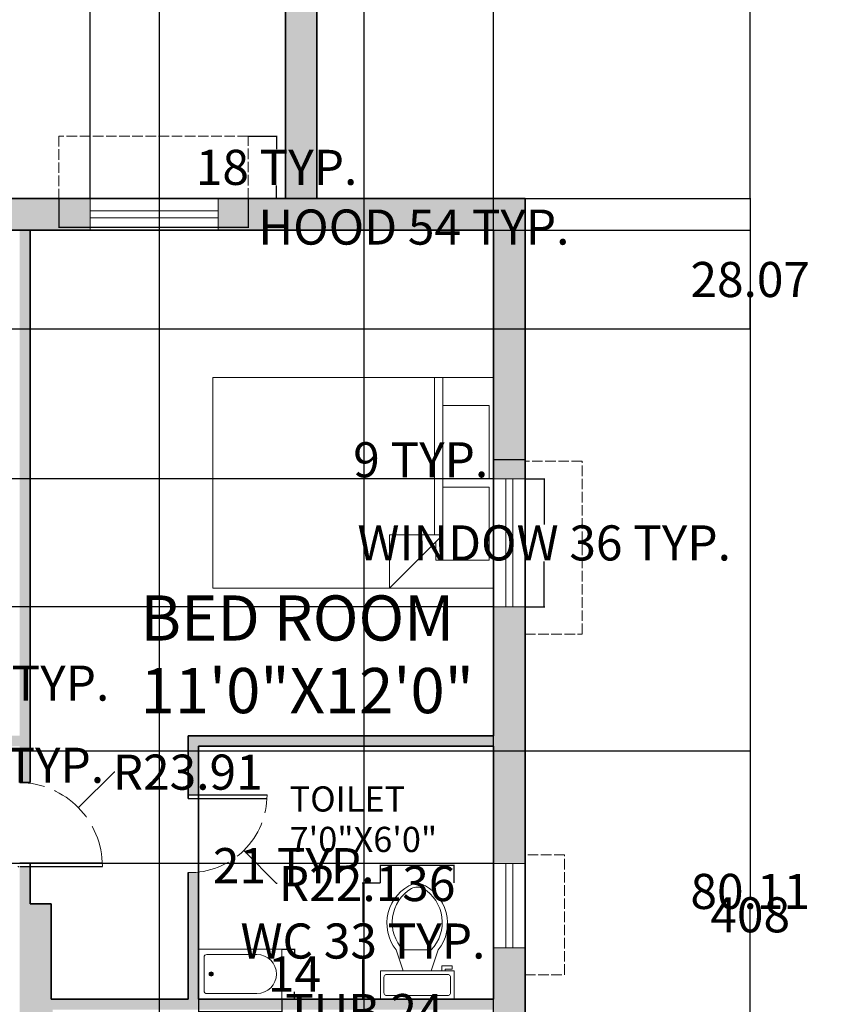
# Model space of a CAD drawing. Units: inches. Extents: x 300 to 1007, y 2 to 1069.
# Tile 7 of 12: x 766 to 995, y 253 to 533. Entities that reach past the tile are written whole.
import ezdxf

# ---------------------------------------------------------------- set-up
doc = ezdxf.new("R2010")
doc.units = ezdxf.units.IN
doc.header["$MEASUREMENT"] = 0
doc.linetypes.add('ACAD_ISO02W100', pattern=[15, 12, -3])
for name, color, linetype, lineweight in [('A-ANNO-DIMS', 2, 'Continuous', 18), ('A-AREA-IDEN', 7, 'Continuous', 18), ('A-DOOR', 3, 'Continuous', 25), ('A-DOOR-SWNG', 3, 'ACAD_ISO02W100', 13), ('A-FLOR-FIXT', 9, 'Continuous', 18), ('A-FLOR-SLAB', 7, 'Continuous', 35), ('A-FURN', 8, 'Continuous', 18), ('A-GLAZ', 4, 'Continuous', 18), ('A-GLAZ-OVHD', 8, 'ACAD_ISO02W100', 13), ('A-WALL', 7, 'Continuous', 35)]:
    doc.layers.add(name, color=color, linetype=linetype, lineweight=lineweight)
doc.layers.add('A-WALL-PATT', color=9, linetype='Continuous', lineweight=9, true_color=0xc7c8ca)
doc.styles.get("Standard").update_dxf_attribs({"font": 'arial.ttf'})
doc.dimstyles.get("Standard").update_dxf_attribs({"dimtxt": 10, "dimasz": 0.18, "dimexe": 0.18, "dimexo": 0.0625, "dimgap": 0.09, "dimtad": 0, "dimtih": 1, "dimtoh": 1, "dimdec": 0, "dimzin": 0, "dimdsep": 46, "dimlunit": 3, "dimtxsty": 'Standard', "dimcen": 0.09, "dimadec": 0, "dimazin": 0, "dimtfac": 1, "dimtdec": 0, "dimtofl": 0, "dimtmove": 0, "dimatfit": 3, "dimfxl": 1, "dimtolj": 1, "dimtzin": 0, "dimarcsym": 0})

# ---------------------------------------------------------------- blocks, each defined once
blk = doc.blocks.new('Bed - Queen')
for p, q in [((0, -80.00003), (0, 0)), ((0, 0), (59.99999, 0)), ((59.99999, 0), (59.99999, -80.00003)), ((7.99999, -1.2), (28.79998, -1.2)), ((7.99999, -14.4), (7.99999, -1.2)), ((28.79998, -1.2), (28.79998, -14.4)), ((31.19999, -1.2), (51.99999, -1.2)), ((31.19999, -14.4), (31.19999, -1.2)), ((51.99999, -1.2), (51.99999, -16.4)), ((0, -14.4), (44.8, -14.4)), ((44.8, -16.8), (0, -16.8)), ((59.99999, -29.6), (44.8, -14.4)), ((44.8, -14.4), (44.8, -29.6)), ((51.99999, -16.4), (46.79936, -16.4)), ((44.8, -29.6), (59.99999, -29.6)), ((59.99999, -80.00003), (0, -80.00003))]:
    blk.add_line(p, q)
blk = doc.blocks.new('Toilet - top')
for p, q in [((9.5, -6), (9.5, -2)), ((-8, -8.5), (-8, -8)), ((-7, -8), (-7, -9.5)), ((-4, -8), (-6, -14)), ((4, -8), (6, -14)), ((-10, -8.5), (-8, -8.5)), ((-10, -9.5), (-10, -8.5)), ((-7, -9.5), (-10, -9.5)), ((4, -14), (-4, -14))]:
    blk.add_line(p, q)
blk.add_lwpolyline([(10.5, -8), (10.5, 0), (-10.5, 0), (-10.5, -8)], close=True)
for points in [[(-9.5, -2), (-9.5, -6)], [(8.5, -1), (-8.5, -1)], [(-8.5, -7), (8.5, -7)]]:
    blk.add_lwpolyline(points)
for centre, radius, start, end in [((-8.62, -1.88), 0.884, 81.8699, 188.1301), ((8.62, -1.88), 0.884, 351.8699, 98.1301), ((-8.62, -6.12), 0.884, 171.8699, 278.1301), ((8.62, -6.12), 0.884, 261.8699, 8.1301), ((3.52, -21.58), 12.17, 141.4691, 247.9714), ((4.2, -21.82), 11.33, 136.3677, 238.9468), ((-3.52, -21.58), 12.17, 292.0284, 38.5307), ((-4.2, -21.82), 11.33, 301.053, 43.6321), ((0, -27.88), 4, 245.7318, 294.2682), ((0, -29), 4, 254.8605, 285.1395)]:
    blk.add_arc(centre, radius, start, end)
blk = doc.blocks.new('Bath Tub - 26 x 60 in.')
for p, q in [((8, -18), (10, -18)), ((9, -17), (9, -19))]:
    blk.add_line(p, q)
blk.add_lwpolyline([(0, -36), (0, 0), (60, 0), (60, -36)], close=True)
for points in [[(4, -30), (4, -6)], [(6, -4), (42, -4)], [(42, -32), (6, -32)]]:
    blk.add_lwpolyline(points)
for radius in [1.5, 1]:
    blk.add_circle((9, -18), radius)
for centre, radius, start, end in [((5.75, -5.75), 1.77, 81.8699, 188.1301), ((42, -18), 14, 270, 90), ((5.75, -30.25), 1.77, 171.8699, 278.1301)]:
    blk.add_arc(centre, radius, start, end)
blk = doc.blocks.new('WIN-24')
for p, q in [((0, -4.5), (0, 4.5)), ((23.96, 0), (23.96, 4.5)), ((23.96, 4.5), (23.96, -4.5)), ((0, 1), (23.96, 1)), ((0, -1), (23.96, -1))]:
    blk.add_line(p, q)
blk = doc.blocks.new('WIN-36_1-2')
for p, q in [((0, 4.5), (0, -4.5)), ((36.49, 0), (36.49, 4.5)), ((36.49, 4.5), (36.49, -4.5)), ((0, 1), (36.49, 1)), ((0, -1), (36.49, -1))]:
    blk.add_line(p, q)
blk = doc.blocks.new('WINDOW-HOOD-54')
at = {"ltscale": 0.25}
for p, q in [((0, 17.83), (-53.97, 17.83)), ((-53.97, 17.83), (-53.97, 0)), ((0, 0), (0, 17.83))]:
    blk.add_line(p, q, dxfattribs=at)
blk = doc.blocks.new('*D27')
at = {"layer": 'A-ANNO-DIMS', "color": 0, "lineweight": -2, "transparency": 16777216}
for p, q in [((777.25, 482.32), (777.25, 474.11)), ((831.22, 482.32), (831.22, 474.11)), ((777.43, 474.29), (831.04, 474.29)), ((831.22, 474.29), (831.4, 474.29))]:
    blk.add_line(p, q, dxfattribs=at)
at = {"layer": 'A-ANNO-DIMS', "color": 0, "transparency": 16777216}
for points in [[(777.43, 474.32), (777.43, 474.26), (777.25, 474.29)], [(831.04, 474.32), (831.04, 474.26), (831.22, 474.29)]]:
    blk.add_solid(points, dxfattribs=at)
at = {"layer": 'Defpoints', "color": 0, "transparency": 16777216}
for p in [(777.25, 482.38), (831.22, 482.38), (831.22, 474.29)]:
    blk.add_point(p, dxfattribs=at)
at = {"layer": 'A-ANNO-DIMS', "color": 0, "transparency": 16777216, "insert": (878.45, 474.29), "char_height": 10, "attachment_point": 5}
blk.add_mtext('\\A1;HOOD 54 TYP.', dxfattribs=at)
blk = doc.blocks.new('*D28')
at = {"layer": 'A-ANNO-DIMS', "color": 0, "lineweight": -2, "transparency": 16777216}
for p, q in [((831.28, 500.22), (839.5, 500.22)), ((839.32, 500.04), (839.32, 496.5)), ((839.32, 482.56), (839.32, 486.1)), ((831.28, 482.38), (839.5, 482.38))]:
    blk.add_line(p, q, dxfattribs=at)
at = {"layer": 'A-ANNO-DIMS', "color": 0, "transparency": 16777216}
for points in [[(839.29, 500.04), (839.35, 500.04), (839.32, 500.22)], [(839.29, 482.56), (839.35, 482.56), (839.32, 482.38)]]:
    blk.add_solid(points, dxfattribs=at)
at = {"layer": 'Defpoints', "color": 0, "transparency": 16777216}
for p in [(831.22, 500.22), (839.32, 500.22), (831.22, 482.38)]:
    blk.add_point(p, dxfattribs=at)
at = {"layer": 'A-ANNO-DIMS', "color": 0, "transparency": 16777216, "insert": (839.32, 491.3), "char_height": 10, "attachment_point": 5}
blk.add_mtext('\\A1;18 TYP.', dxfattribs=at)
blk = doc.blocks.new('*D31')
at = {"layer": 'A-ANNO-DIMS', "color": 0, "lineweight": -2, "transparency": 16777216}
for p, q in [((868.84, 287.43), (863.76, 287.43)), ((863.94, 287.25), (863.94, 276.17)), ((863.94, 254.56), (863.94, 265.64)), ((868.84, 254.38), (863.76, 254.38))]:
    blk.add_line(p, q, dxfattribs=at)
at = {"layer": 'A-ANNO-DIMS', "color": 0, "transparency": 16777216}
for points in [[(863.91, 287.25), (863.97, 287.25), (863.94, 287.43)], [(863.91, 254.56), (863.97, 254.56), (863.94, 254.38)]]:
    blk.add_solid(points, dxfattribs=at)
at = {"layer": 'Defpoints', "color": 0, "transparency": 16777216}
for p in [(868.9, 287.43), (863.94, 254.38), (868.9, 254.38)]:
    blk.add_point(p, dxfattribs=at)
at = {"layer": 'A-ANNO-DIMS', "color": 0, "transparency": 16777216, "insert": (863.94, 270.91), "char_height": 10, "attachment_point": 5}
blk.add_mtext('\\A1;WC 33 TYP.', dxfattribs=at)
blk = doc.blocks.new('*D32')
at = {"layer": 'A-ANNO-DIMS', "color": 0, "lineweight": -2, "transparency": 16777216}
for p, q in [((868.9, 292.39), (868.72, 292.39)), ((868.9, 287.49), (868.9, 292.57)), ((889.72, 292.39), (869.08, 292.39)), ((889.9, 287.49), (889.9, 292.57))]:
    blk.add_line(p, q, dxfattribs=at)
at = {"layer": 'A-ANNO-DIMS', "color": 0, "transparency": 16777216}
for points in [[(869.08, 292.42), (869.08, 292.36), (868.9, 292.39)], [(889.72, 292.42), (889.72, 292.36), (889.9, 292.39)]]:
    blk.add_solid(points, dxfattribs=at)
at = {"layer": 'Defpoints', "color": 0, "transparency": 16777216}
for p in [(868.9, 292.39), (868.9, 287.43), (889.9, 287.43)]:
    blk.add_point(p, dxfattribs=at)
at = {"layer": 'A-ANNO-DIMS', "color": 0, "transparency": 16777216, "insert": (844.2, 292.39), "char_height": 10, "attachment_point": 5}
blk.add_mtext('\\A1;21 TYP.', dxfattribs=at)
blk = doc.blocks.new('*D37')
at = {"layer": 'A-ANNO-DIMS', "color": 0, "lineweight": -2, "transparency": 16777216}
for p, q in [((817.12, 254.32), (817.12, 250.64)), ((840.87, 254.32), (840.87, 250.64)), ((817.3, 250.82), (840.69, 250.82)), ((840.87, 250.82), (841.05, 250.82))]:
    blk.add_line(p, q, dxfattribs=at)
at = {"layer": 'A-ANNO-DIMS', "color": 0, "transparency": 16777216}
for points in [[(817.3, 250.85), (817.3, 250.79), (817.12, 250.82)], [(840.69, 250.85), (840.69, 250.79), (840.87, 250.82)]]:
    blk.add_solid(points, dxfattribs=at)
at = {"layer": 'Defpoints', "color": 0, "transparency": 16777216}
for p in [(817.12, 254.38), (840.87, 254.38), (840.87, 250.82)]:
    blk.add_point(p, dxfattribs=at)
at = {"layer": 'A-ANNO-DIMS', "color": 0, "transparency": 16777216, "insert": (864.32, 250.82), "char_height": 10, "attachment_point": 5}
blk.add_mtext('\\A1;TUB 24', dxfattribs=at)
blk = doc.blocks.new('*D38')
at = {"layer": 'A-ANNO-DIMS', "color": 0, "lineweight": -2, "transparency": 16777216}
for p, q in [((840.93, 268.63), (844.61, 268.63)), ((844.43, 268.45), (844.43, 266.62)), ((844.43, 254.56), (844.43, 256.4)), ((840.93, 254.38), (844.61, 254.38))]:
    blk.add_line(p, q, dxfattribs=at)
at = {"layer": 'A-ANNO-DIMS', "color": 0, "transparency": 16777216}
for points in [[(844.4, 268.45), (844.46, 268.45), (844.43, 268.63)], [(844.4, 254.56), (844.46, 254.56), (844.43, 254.38)]]:
    blk.add_solid(points, dxfattribs=at)
at = {"layer": 'Defpoints', "color": 0, "transparency": 16777216}
for p in [(840.87, 268.63), (844.43, 268.63), (840.87, 254.38)]:
    blk.add_point(p, dxfattribs=at)
at = {"layer": 'A-ANNO-DIMS', "color": 0, "transparency": 16777216, "insert": (844.43, 261.51), "char_height": 10, "attachment_point": 5}
blk.add_mtext('\\A1;14', dxfattribs=at)
blk = doc.blocks.new('*D59')
at = {"layer": 'A-ANNO-DIMS', "color": 0, "lineweight": -2, "transparency": 16777216}
for p, q in [((910.18, 402.54), (915.77, 402.54)), ((915.59, 402.36), (915.59, 389.59)), ((915.59, 366.28), (915.59, 379.05)), ((910.18, 366.1), (915.77, 366.1))]:
    blk.add_line(p, q, dxfattribs=at)
at = {"layer": 'A-ANNO-DIMS', "color": 0, "transparency": 16777216}
for points in [[(915.56, 402.36), (915.62, 402.36), (915.59, 402.54)], [(915.56, 366.28), (915.62, 366.28), (915.59, 366.1)]]:
    blk.add_solid(points, dxfattribs=at)
at = {"layer": 'Defpoints', "color": 0, "transparency": 16777216}
for p in [(910.12, 402.54), (915.59, 402.54), (910.12, 366.1)]:
    blk.add_point(p, dxfattribs=at)
at = {"layer": 'A-ANNO-DIMS', "color": 0, "transparency": 16777216, "insert": (915.59, 384.32), "char_height": 10, "attachment_point": 5}
blk.add_mtext('\\A1;WINDOW 36 TYP.', dxfattribs=at)
blk = doc.blocks.new('*D60')
at = {"layer": 'A-ANNO-DIMS', "color": 0, "lineweight": -2, "transparency": 16777216}
for p, q in [((901.12, 408), (900.94, 408)), ((901.12, 402.6), (901.12, 408.18)), ((909.94, 408), (901.3, 408)), ((910.12, 402.6), (910.12, 408.18))]:
    blk.add_line(p, q, dxfattribs=at)
at = {"layer": 'A-ANNO-DIMS', "color": 0, "transparency": 16777216}
for points in [[(901.3, 408.03), (901.3, 407.97), (901.12, 408)], [(909.94, 408.03), (909.94, 407.97), (910.12, 408)]]:
    blk.add_solid(points, dxfattribs=at)
at = {"layer": 'Defpoints', "color": 0, "transparency": 16777216}
for p in [(901.12, 408), (901.12, 402.54), (910.12, 402.54)]:
    blk.add_point(p, dxfattribs=at)
at = {"layer": 'A-ANNO-DIMS', "color": 0, "transparency": 16777216, "insert": (880.4, 408), "char_height": 10, "attachment_point": 5}
blk.add_mtext('\\A1;9 TYP.', dxfattribs=at)
blk = doc.blocks.new('*D65')
at = {"layer": 'A-ANNO-DIMS', "color": 0, "lineweight": -2, "transparency": 16777216}
for p, q in [((742.62, 362.38), (748.14, 362.38)), ((747.96, 362.2), (747.96, 349.65)), ((747.96, 326.56), (747.96, 339.12)), ((742.62, 326.38), (748.14, 326.38))]:
    blk.add_line(p, q, dxfattribs=at)
at = {"layer": 'A-ANNO-DIMS', "color": 0, "transparency": 16777216}
for points in [[(747.93, 362.2), (747.99, 362.2), (747.96, 362.38)], [(747.93, 326.56), (747.99, 326.56), (747.96, 326.38)]]:
    blk.add_solid(points, dxfattribs=at)
at = {"layer": 'Defpoints', "color": 0, "transparency": 16777216}
for p in [(742.56, 362.38), (747.96, 362.38), (742.56, 326.38)]:
    blk.add_point(p, dxfattribs=at)
at = {"layer": 'A-ANNO-DIMS', "color": 0, "transparency": 16777216, "insert": (747.96, 344.38), "char_height": 10, "attachment_point": 5}
blk.add_mtext('\\A1;DOOR 36 TYP.', dxfattribs=at)
blk = doc.blocks.new('*D66')
at = {"layer": 'A-ANNO-DIMS', "color": 0, "lineweight": -2, "transparency": 16777216}
for p, q in [((706.81, 326.32), (706.81, 320.8)), ((742.56, 326.32), (742.56, 320.8)), ((706.99, 320.98), (742.38, 320.98)), ((742.56, 320.98), (742.74, 320.98))]:
    blk.add_line(p, q, dxfattribs=at)
at = {"layer": 'A-ANNO-DIMS', "color": 0, "transparency": 16777216}
for points in [[(706.99, 321.01), (706.99, 320.95), (706.81, 320.98)], [(742.38, 321.01), (742.38, 320.95), (742.56, 320.98)]]:
    blk.add_solid(points, dxfattribs=at)
at = {"layer": 'Defpoints', "color": 0, "transparency": 16777216}
for p in [(706.81, 326.38), (742.56, 326.38), (742.56, 320.98)]:
    blk.add_point(p, dxfattribs=at)
at = {"layer": 'A-ANNO-DIMS', "color": 0, "transparency": 16777216, "insert": (767.16, 320.98), "char_height": 10, "attachment_point": 5}
blk.add_mtext('\\A1;36 TYP.', dxfattribs=at)
blk = doc.blocks.new('*D76')
at = {"layer": 'A-ANNO-DIMS', "color": 0, "lineweight": -2, "transparency": 16777216}
for p, q in [((910.18, 482.38), (974.48, 482.38)), ((974.3, 482.2), (974.3, 283.58)), ((974.3, 74.56), (974.3, 273.19)), ((910.18, 74.38), (974.48, 74.38))]:
    blk.add_line(p, q, dxfattribs=at)
at = {"layer": 'A-ANNO-DIMS', "color": 0, "transparency": 16777216}
for points in [[(974.27, 482.2), (974.33, 482.2), (974.3, 482.38)], [(974.27, 74.56), (974.33, 74.56), (974.3, 74.38)]]:
    blk.add_solid(points, dxfattribs=at)
at = {"layer": 'Defpoints', "color": 0, "transparency": 16777216}
for p in [(910.12, 482.38), (974.3, 482.38), (910.12, 74.38)]:
    blk.add_point(p, dxfattribs=at)
at = {"layer": 'A-ANNO-DIMS', "color": 0, "transparency": 16777216, "insert": (974.3, 278.38), "char_height": 10, "attachment_point": 5}
blk.add_mtext('\\A1;408', dxfattribs=at)
blk = doc.blocks.new('*D77')
at = {"layer": 'A-ANNO-DIMS', "color": 0, "lineweight": -2, "transparency": 16777216}
for p, q in [((841.89, 609.45), (974.48, 609.45)), ((974.3, 609.27), (974.3, 551.11)), ((974.3, 482.56), (974.3, 540.72)), ((850.89, 482.38), (974.48, 482.38))]:
    blk.add_line(p, q, dxfattribs=at)
at = {"layer": 'A-ANNO-DIMS', "color": 0, "transparency": 16777216}
for points in [[(974.27, 609.27), (974.33, 609.27), (974.3, 609.45)], [(974.27, 482.56), (974.33, 482.56), (974.3, 482.38)]]:
    blk.add_solid(points, dxfattribs=at)
at = {"layer": 'Defpoints', "color": 0, "transparency": 16777216}
for p in [(841.83, 609.45), (974.3, 609.45), (850.83, 482.38)]:
    blk.add_point(p, dxfattribs=at)
at = {"layer": 'A-ANNO-DIMS', "color": 0, "transparency": 16777216, "insert": (974.3, 545.92), "char_height": 10, "attachment_point": 5}
blk.add_mtext('\\A1;127.06', dxfattribs=at)
blk = doc.blocks.new('*D84')
at = {"layer": 'A-ANNO-DIMS', "color": 0, "lineweight": -2, "transparency": 16777216}
for p, q in [((864.25, 225.89), (864.25, 1063.03)), ((901.12, 225.89), (901.12, 1063.03)), ((864.43, 1062.85), (865.73, 1062.85)), ((900.94, 1062.85), (899.65, 1062.85))]:
    blk.add_line(p, q, dxfattribs=at)
at = {"layer": 'A-ANNO-DIMS', "color": 0, "transparency": 16777216}
for points in [[(864.43, 1062.88), (864.43, 1062.82), (864.25, 1062.85)], [(900.94, 1062.88), (900.94, 1062.82), (901.12, 1062.85)]]:
    blk.add_solid(points, dxfattribs=at)
at = {"layer": 'Defpoints', "color": 0, "transparency": 16777216}
for p in [(901.12, 1062.85), (864.25, 225.83), (901.12, 225.83)]:
    blk.add_point(p, dxfattribs=at)
at = {"layer": 'A-ANNO-DIMS', "color": 0, "transparency": 16777216, "insert": (882.69, 1062.85), "char_height": 10, "attachment_point": 5}
blk.add_mtext('\\A1;36.87', dxfattribs=at)
blk = doc.blocks.new('*D86')
at = {"layer": 'A-ANNO-DIMS', "color": 0, "lineweight": -2, "transparency": 16777216}
for p, q in [((805.95, 235.15), (805.95, 1063.03)), ((864.25, 235.15), (864.25, 1063.03)), ((806.13, 1062.85), (822.02, 1062.85)), ((864.07, 1062.85), (848.18, 1062.85))]:
    blk.add_line(p, q, dxfattribs=at)
at = {"layer": 'A-ANNO-DIMS', "color": 0, "transparency": 16777216}
for points in [[(806.13, 1062.88), (806.13, 1062.82), (805.95, 1062.85)], [(864.07, 1062.88), (864.07, 1062.82), (864.25, 1062.85)]]:
    blk.add_solid(points, dxfattribs=at)
at = {"layer": 'Defpoints', "color": 0, "transparency": 16777216}
for p in [(864.25, 1062.85), (805.95, 235.08), (864.25, 235.08)]:
    blk.add_point(p, dxfattribs=at)
at = {"layer": 'A-ANNO-DIMS', "color": 0, "transparency": 16777216, "insert": (835.1, 1062.85), "char_height": 10, "attachment_point": 5}
blk.add_mtext('\\A1;58.3', dxfattribs=at)
blk = doc.blocks.new('*D91')
at = {"layer": 'A-ANNO-DIMS', "color": 0, "lineweight": -2, "transparency": 16777216}
for p, q in [((429.18, 325.09), (974.48, 325.09)), ((974.3, 324.91), (974.3, 290.23)), ((974.3, 245.16), (974.3, 279.84)), ((429.18, 244.98), (974.48, 244.98))]:
    blk.add_line(p, q, dxfattribs=at)
at = {"layer": 'A-ANNO-DIMS', "color": 0, "transparency": 16777216}
for points in [[(974.27, 324.91), (974.33, 324.91), (974.3, 325.09)], [(974.27, 245.16), (974.33, 245.16), (974.3, 244.98)]]:
    blk.add_solid(points, dxfattribs=at)
at = {"layer": 'Defpoints', "color": 0, "transparency": 16777216}
for p in [(429.12, 325.09), (974.3, 325.09), (429.12, 244.98)]:
    blk.add_point(p, dxfattribs=at)
at = {"layer": 'A-ANNO-DIMS', "color": 0, "transparency": 16777216, "insert": (974.3, 285.04), "char_height": 10, "attachment_point": 5}
blk.add_mtext('\\A1;80.11', dxfattribs=at)
blk = doc.blocks.new('*D92')
at = {"layer": 'A-ANNO-DIMS', "color": 0, "lineweight": -2, "transparency": 16777216}
for p, q in [((429.18, 473.38), (974.48, 473.38)), ((974.3, 473.2), (974.3, 464.54)), ((974.3, 445.49), (974.3, 454.15)), ((429.18, 445.31), (974.48, 445.31))]:
    blk.add_line(p, q, dxfattribs=at)
at = {"layer": 'A-ANNO-DIMS', "color": 0, "transparency": 16777216}
for points in [[(974.27, 473.2), (974.33, 473.2), (974.3, 473.38)], [(974.27, 445.49), (974.33, 445.49), (974.3, 445.31)]]:
    blk.add_solid(points, dxfattribs=at)
at = {"layer": 'Defpoints', "color": 0, "transparency": 16777216}
for p in [(429.12, 473.38), (429.12, 445.31), (974.3, 445.31)]:
    blk.add_point(p, dxfattribs=at)
at = {"layer": 'A-ANNO-DIMS', "color": 0, "transparency": 16777216, "insert": (974.3, 459.35), "char_height": 10, "attachment_point": 5}
blk.add_mtext('\\A1;28.07', dxfattribs=at)
blk = doc.blocks.new('*D95')
at = {"layer": 'A-ANNO-DIMS', "color": 0, "lineweight": -2, "transparency": 16777216}
for p, q in [((901.06, 473.38), (354.19, 473.38)), ((354.37, 473.2), (354.37, 443.16)), ((354.37, 402.72), (354.37, 432.77)), ((901.06, 402.54), (354.19, 402.54))]:
    blk.add_line(p, q, dxfattribs=at)
at = {"layer": 'A-ANNO-DIMS', "color": 0, "transparency": 16777216}
for points in [[(354.34, 473.2), (354.4, 473.2), (354.37, 473.38)], [(354.34, 402.72), (354.4, 402.72), (354.37, 402.54)]]:
    blk.add_solid(points, dxfattribs=at)
at = {"layer": 'Defpoints', "color": 0, "transparency": 16777216}
for p in [(354.37, 473.38), (901.12, 473.38), (901.12, 402.54)]:
    blk.add_point(p, dxfattribs=at)
at = {"layer": 'A-ANNO-DIMS', "color": 0, "transparency": 16777216, "insert": (354.37, 437.96), "char_height": 10, "attachment_point": 5}
blk.add_mtext('\\A1;70.85', dxfattribs=at)
blk = doc.blocks.new('*D96')
at = {"layer": 'A-ANNO-DIMS', "color": 0, "lineweight": -2, "transparency": 16777216}
for p, q in [((901.06, 366.1), (354.19, 366.1)), ((354.37, 365.92), (354.37, 334.77)), ((354.37, 293.21), (354.37, 324.37)), ((901.06, 293.03), (354.19, 293.03))]:
    blk.add_line(p, q, dxfattribs=at)
at = {"layer": 'A-ANNO-DIMS', "color": 0, "transparency": 16777216}
for points in [[(354.34, 365.92), (354.4, 365.92), (354.37, 366.1)], [(354.34, 293.21), (354.4, 293.21), (354.37, 293.03)]]:
    blk.add_solid(points, dxfattribs=at)
at = {"layer": 'Defpoints', "color": 0, "transparency": 16777216}
for p in [(354.37, 366.1), (901.12, 366.1), (901.12, 293.03)]:
    blk.add_point(p, dxfattribs=at)
at = {"layer": 'A-ANNO-DIMS', "color": 0, "transparency": 16777216, "insert": (354.37, 329.57), "char_height": 10, "attachment_point": 5}
blk.add_mtext('\\A1;73.07', dxfattribs=at)
blk = doc.blocks.new('*D100')
at = {"layer": 'A-ANNO-DIMS', "color": 0, "lineweight": -2, "transparency": 16777216}
for p, q in [((716.78, 482.45), (716.78, 1063.03)), ((786.22, 482.45), (786.22, 1063.03)), ((716.96, 1062.85), (734.53, 1062.85)), ((786.04, 1062.85), (768.47, 1062.85))]:
    blk.add_line(p, q, dxfattribs=at)
at = {"layer": 'A-ANNO-DIMS', "color": 0, "transparency": 16777216}
for points in [[(716.96, 1062.88), (716.96, 1062.82), (716.78, 1062.85)], [(786.04, 1062.88), (786.04, 1062.82), (786.22, 1062.85)]]:
    blk.add_solid(points, dxfattribs=at)
at = {"layer": 'Defpoints', "color": 0, "transparency": 16777216}
for p in [(786.22, 1062.85), (716.78, 482.38), (786.22, 482.38)]:
    blk.add_point(p, dxfattribs=at)
at = {"layer": 'A-ANNO-DIMS', "color": 0, "transparency": 16777216, "insert": (751.5, 1062.85), "char_height": 10, "attachment_point": 5}
blk.add_mtext('\\A1;69.44', dxfattribs=at)
blk = doc.blocks.new('*D119')
at = {"layer": 'A-ANNO-DIMS', "color": 0, "lineweight": -2, "transparency": 16777216}
for p, q in [((793.02, 319.02), (782.94, 309.07)), ((793.2, 319.02), (793.02, 319.02)), ((765.69, 292.16), (765.87, 292.16)), ((765.78, 292.07), (765.78, 292.25))]:
    blk.add_line(p, q, dxfattribs=at)
at = {"layer": 'A-ANNO-DIMS', "color": 0, "transparency": 16777216}
blk.add_solid([(782.92, 309.09), (782.96, 309.05), (782.81, 308.94)], dxfattribs=at)
at = {"layer": 'Defpoints', "color": 0, "transparency": 16777216}
for p in [(782.81, 308.94), (765.78, 292.16)]:
    blk.add_point(p, dxfattribs=at)
at = {"layer": 'A-ANNO-DIMS', "color": 0, "transparency": 16777216, "insert": (813.99, 319.02), "char_height": 10, "attachment_point": 5}
blk.add_mtext('\\A1;R23.91', dxfattribs=at)
blk = doc.blocks.new('*D120')
at = {"layer": 'A-ANNO-DIMS', "color": 0, "lineweight": -2, "transparency": 16777216}
for p, q in [((814.38, 312.52), (814.56, 312.52)), ((814.47, 312.43), (814.47, 312.61)), ((839.32, 287.28), (830.13, 296.61)), ((839.5, 287.28), (839.32, 287.28))]:
    blk.add_line(p, q, dxfattribs=at)
at = {"layer": 'A-ANNO-DIMS', "color": 0, "transparency": 16777216}
blk.add_solid([(830.15, 296.63), (830.1, 296.59), (830, 296.74)], dxfattribs=at)
at = {"layer": 'Defpoints', "color": 0, "transparency": 16777216}
for p in [(814.47, 312.52), (830, 296.74)]:
    blk.add_point(p, dxfattribs=at)
at = {"layer": 'A-ANNO-DIMS', "color": 0, "transparency": 16777216, "insert": (865.13, 287.28), "char_height": 10, "attachment_point": 5}
blk.add_mtext('\\A1;R22.136', dxfattribs=at)

msp = doc.modelspace()

# ---------------------------------------------------------------- hatches: boundary and pattern name
at = {"layer": 'A-WALL-PATT'}
h = msp.add_hatch(color=256, dxfattribs=at)
h.dxf.hatch_style = 1
h.paths.add_polyline_path([(546.104, 999.4468), (478.8267, 999.4468), (478.8267, 869.2798, -0.06322715), (487.8267, 868.1328), (487.8267, 990.4468), (546.104, 990.4468)])
h.paths.add_polyline_path([(630.4852, 999.4468), (582.106, 999.4468), (582.106, 990.4468), (613.8267, 990.4468), (613.8267, 867.4468), (622.8267, 867.4468), (622.8267, 990.4468), (630.4852, 990.4468)])
h.paths.add_polyline_path([(702.0883, 999.4468), (650.4653, 999.4468), (650.4653, 990.4468), (682.8267, 990.4468), (682.8267, 960.0824, -0.02530575), (685.8267, 960.0478), (685.8267, 990.4468), (702.0883, 990.4468)])
h.paths.add_polyline_path([(850.8267, 999.4468), (737.5888, 999.4468), (737.5888, 990.4468), (841.8267, 990.4468), (841.8267, 950.5685), (850.8267, 950.5685)])
h.paths.add_polyline_path([(685.8267, 930.4465), (682.8267, 930.4465), (682.8267, 888.4468), (682.8267, 867.4468), (685.8267, 867.4468), (697.4169, 867.4468), (697.4169, 870.4468), (685.8267, 870.4468), (685.8267, 888.4468)])
h.paths.add_polyline_path([(682.8267, 931.4465), (654.3436, 931.4465, 0.00843109), (654.3267, 930.4465), (682.8267, 930.4465)])
h.paths.add_polyline_path([(685.8267, 931.4465), (682.8267, 931.4465), (682.8267, 930.4465), (685.8267, 930.4465)])
h.paths.add_polyline_path([(682.8267, 888.4468), (622.8267, 888.4468), (622.8267, 885.4468), (682.8267, 885.4468)])
h.paths.add_polyline_path([(850.8267, 870.4468), (850.8267, 914.7851), (841.8267, 914.7851), (841.8267, 870.4468), (732.7101, 870.4468, -0.02120595), (732.8267, 867.4468), (779.8267, 867.4468), (779.8267, 749.4468), (782.8267, 749.4468), (788.8267, 749.4468), (788.8267, 861.4468), (841.8267, 861.4468), (841.8267, 749.4468), (850.8267, 749.4468)])
h.paths.add_polyline_path([(622.8267, 810.4468), (487.8267, 810.4468), (487.8267, 833.2626), (478.8267, 833.2626), (478.8267, 609.4468), (478.8267, 482.3847), (487.8267, 482.3847), (487.8267, 801.4468), (620.8267, 801.4468), (622.8267, 801.4468)])
h.paths.add_polyline_path([(680.8267, 729.4468), (620.8267, 729.4468), (620.8267, 765.8246, -0.02111352), (617.8267, 766.0562), (617.8267, 698.7303), (620.8267, 698.7303), (620.8267, 726.4468), (680.8267, 726.4468)])
h.paths.add_polyline_path([(620.8267, 668.8122, -0.02498293), (617.8267, 668.6448), (617.8267, 618.4468), (600.3357, 618.4468), (600.3357, 609.4468), (652.9929, 609.4468), (652.9929, 618.4468), (620.8267, 618.4468)])
h.paths.add_polyline_path([(552.3393, 618.4468), (487.8267, 618.4468), (487.8267, 609.4468), (552.3393, 609.4468)], flags=17)
h.paths.add_polyline_path([(694.5763, 618.4468), (683.8267, 618.4468), (683.8267, 726.4468), (683.8267, 749.4468), (680.8267, 749.4468), (680.8267, 740.4468), (680.8267, 726.4468), (680.8267, 618.4468), (674.1573, 618.4468), (674.1573, 609.4468), (680.8267, 609.4468), (694.5763, 609.4468)])
h.paths.add_polyline_path([(850.8267, 642.8902), (841.8267, 642.8902), (841.8267, 618.4468), (782.8267, 618.4468), (782.8267, 708.0513, -0.02308839), (779.8267, 707.9092), (779.8267, 618.4468), (730.1068, 618.4468), (730.1068, 609.4468), (779.8267, 609.4468), (841.8267, 609.4468), (841.8267, 482.3847), (850.8267, 482.3847)])
h.paths.add_polyline_path([(850.8267, 749.4468), (841.8267, 749.4468), (841.8267, 705.9119), (850.8267, 705.9119)])
h.paths.add_polyline_path([(841.8267, 749.4468), (782.8267, 749.4468), (779.8267, 749.4468), (761.9959, 749.4468), (761.9959, 740.4468), (779.8267, 740.4468), (812.3267, 740.4468), (841.8267, 740.4468)])
h.paths.add_polyline_path([(669.1457, 482.3847), (604.489, 482.3847), (604.489, 473.3847), (631.1217, 473.3847), (631.1217, 436.0244, -0.02504709), (634.1217, 436.1748), (634.1217, 436.4367), (634.1217, 473.3847), (669.1457, 473.3847)], flags=17)
h.paths.add_polyline_path([(580.5305, 482.3847), (571.1217, 482.3847), (541.0813, 482.3847), (541.0813, 473.3847), (562.1217, 473.3847), (562.1217, 326.3847), (571.1217, 326.3847), (571.1217, 362.3847), (631.1217, 362.3847), (631.1217, 326.3847), (706.9024, 326.3847, -0.02105388), (706.9999, 329.3847), (634.1217, 329.3847), (634.1217, 365.3847), (634.1217, 406.1748), (631.1217, 406.1748), (631.1217, 365.3847), (571.1217, 365.3847), (571.1217, 473.3847), (580.5305, 473.3847)])
h.paths.add_polyline_path([(493.4756, 482.3847), (420.1217, 482.3847), (420.1217, 445.3134), (429.1217, 445.3134), (429.1217, 473.3847), (493.4756, 473.3847)])
h.paths.add_polyline_path([(786.2236, 482.3847), (716.7793, 482.3847), (716.7793, 473.3847), (766.1217, 473.3847), (766.1217, 329.3847), (742.5583, 329.3847), (742.5583, 326.3847), (766.1217, 326.3847), (766.1217, 316.0647), (769.1217, 316.0647), (769.1217, 326.3847), (769.1217, 473.3847), (786.2236, 473.3847)])
h.paths.add_polyline_path([(910.1217, 482.3847), (822.7166, 482.3847), (822.7166, 473.3847), (901.1217, 473.3847), (901.1217, 402.5393), (910.1217, 402.5393)])
h.paths.add_polyline_path([(910.1217, 366.1034), (901.1217, 366.1034), (901.1217, 329.3847), (814.1217, 329.3847), (814.1217, 312.5176), (817.1217, 312.5176), (817.1217, 326.3847), (901.1217, 326.3847), (901.1217, 293.0319), (910.1217, 293.0319), (910.1217, 326.3847)])
h.paths.add_polyline_path([(910.1217, 268.9355), (901.1217, 268.9355), (901.1217, 254.3847), (817.1217, 254.3847), (817.1217, 290.5411, -0.03396715), (814.1217, 290.3847), (814.1217, 254.3847), (775.1217, 254.3847), (775.1217, 281.5164), (769.1217, 281.5164), (769.1217, 292.1577), (766.1217, 292.1577), (766.1217, 254.3847), (766.1217, 220.1938), (775.5079, 220.1938), (775.5079, 251.3847), (817.1217, 251.3847), (901.1217, 251.3847), (901.1217, 152.3847), (819.0246, 152.3847, -0.02493798), (818.9117, 149.3847), (901.1217, 149.3847), (901.1217, 92.3847), (901.1217, 83.3847), (874.3528, 83.3847), (874.3528, 74.3847), (910.1217, 74.3847), (910.1217, 92.3847), (910.1217, 149.3847)])
h.paths.add_polyline_path([(429.1217, 325.0924), (420.1217, 325.0924), (420.1217, 263.3847), (420.1217, 244.9834), (429.1217, 244.9834), (429.1217, 269.3847), (571.1217, 269.3847), (571.1217, 272.3847), (562.1217, 272.3847), (429.1217, 272.3847)])
h.paths.add_polyline_path([(429.1217, 208.998), (420.1217, 208.998), (420.1217, 74.3847), (496.7704, 74.3847), (496.7704, 83.3847), (429.1217, 83.3847)])
h.paths.add_polyline_path([(598.4322, 83.3847), (571.1217, 83.3847), (571.1217, 122.1171), (562.1217, 122.1171), (562.1217, 83.3847), (544.6031, 83.3847), (544.6031, 74.3847), (598.4322, 74.3847)])
h.paths.add_polyline_path([(797.0822, 83.3847), (769.1217, 83.3847), (769.1217, 149.3847), (788.9123, 149.3847), (788.9123, 152.3847), (769.1217, 152.3847), (769.1217, 178.0167), (766.1217, 178.0167), (766.1217, 152.3847), (735.3598, 152.3847), (735.3598, 143.3847), (766.1217, 143.3847), (766.1217, 83.3847), (634.1217, 83.3847), (634.1217, 143.3847), (659.7326, 143.3847), (659.7326, 152.3847), (634.1217, 152.3847), (634.1217, 194.3847), (571.1217, 194.3847), (571.1217, 233.7289, -0.06379947), (562.1217, 234.7942), (562.1217, 163.4485), (567.7403, 163.4485), (567.7403, 152.3847), (571.1217, 152.3847), (571.1217, 191.3847), (631.1217, 191.3847), (631.1217, 83.3847), (621.979, 83.3847), (621.979, 74.3847), (631.1217, 74.3847), (797.0822, 74.3847)])

# ---------------------------------------------------------------- linework, layer by layer
at = {"layer": 'A-DOOR'}
for p, q in [((814.1217, 312.5176), (817.1217, 312.5176)), ((814.1217, 312.5176), (814.1217, 311.5176)), ((814.1217, 312.5176), (836.6078, 312.5176)), ((814.1217, 312.5176), (814.1217, 311.8837)), ((814.1217, 311.8837), (814.1217, 311.5176)), ((814.1217, 311.5176), (836.6078, 311.5176)), ((766.1217, 293.1577), (789.6933, 293.1577)), ((766.1217, 292.1577), (789.6933, 292.1577))]:
    msp.add_line(p, q, dxfattribs=at)
at = {"layer": 'A-DOOR-SWNG'}
for centre, radius, start, end in [((765.784, 292.1577), 23.9093, 0, 89.190772), ((814.4722, 312.5176), 22.1356, 269.092795, 0)]:
    msp.add_arc(centre, radius, start, end, dxfattribs=at)
at = {"layer": 'A-FLOR-SLAB'}
msp.add_line((841.8267, 482.3847), (841.8267, 609.4468), dxfattribs=at)
at = {"layer": 'A-GLAZ-OVHD', "ltscale": 0.25}
for p, q in [((926.3773, 407.5628), (910.1217, 407.5628)), ((926.3773, 358.3615), (926.3773, 407.5628)), ((910.1217, 358.3615), (926.3773, 358.3615)), ((921.415, 295.4755), (910.1217, 295.4755)), ((921.415, 261.2939), (921.415, 295.4755)), ((910.1217, 261.2939), (921.415, 261.2939))]:
    msp.add_line(p, q, dxfattribs=at)
at = {"layer": 'A-WALL'}
for p, q in [((850.8267, 482.3847), (850.8267, 749.4468)), ((571.1217, 482.3847), (910.1217, 482.3847)), ((910.1217, 482.3847), (910.1217, 74.3847)), ((769.1217, 473.3847), (769.1217, 326.3847)), ((769.1217, 473.3847), (901.1217, 473.3847)), ((901.1217, 473.3847), (901.1217, 329.3847)), ((901.1217, 329.3847), (814.1217, 329.3847)), ((814.1217, 311.5176), (814.1217, 329.3847)), ((769.1217, 326.3847), (769.1217, 316.0647)), ((901.1217, 326.3847), (817.1217, 326.3847)), ((817.1217, 254.3847), (817.1217, 326.3847)), ((901.1217, 326.3847), (901.1217, 254.3847)), ((910.1217, 326.3847), (910.1217, 254.3847)), ((769.1217, 316.0647), (766.1217, 316.0647)), ((769.1217, 293.1577), (769.1217, 281.5164)), ((814.1217, 254.3847), (814.1217, 290.3847)), ((775.1217, 281.5164), (769.1217, 281.5164)), ((775.1217, 281.5164), (775.1217, 254.3847)), ((775.1217, 254.3847), (814.1217, 254.3847)), ((901.1217, 254.3847), (817.1217, 254.3847))]:
    msp.add_line(p, q, dxfattribs=at)

# ---------------------------------------------------------------- block references
at = {"layer": 'A-FLOR-FIXT', "rotation": 180}
msp.add_blockref('Toilet - top', (879.3982, 254.3847), dxfattribs=at)
at = {"layer": 'A-FLOR-FIXT', "xscale": 0.395805995043668, "yscale": 0.395805995043668, "zscale": 0.395805995043668}
msp.add_blockref('Bath Tub - 26 x 60 in.', (817.1217, 268.6337), dxfattribs=at)
at = {"layer": 'A-FURN', "rotation": 270}
msp.add_blockref('Bed - Queen', (901.1217, 431.432), dxfattribs=at)
at = {"layer": 'A-GLAZ'}
msp.add_blockref('WIN-36_1-2', (786.2236, 477.8847), dxfattribs=at)
at = {"layer": 'A-GLAZ', "xscale": 0.9984346954045866, "rotation": 90}
msp.add_blockref('WIN-36_1-2', (905.6217, 366.1034), dxfattribs=at)
at = {"layer": 'A-GLAZ', "extrusion": (0, 0, -1), "xscale": 1.005753087191701, "zscale": -1, "rotation": 90}
msp.add_blockref('WIN-24', (-905.6217, 268.9355), dxfattribs=at)
at = {"layer": 'A-GLAZ-OVHD'}
msp.add_blockref('WINDOW-HOOD-54', (831.22, 482.3847), dxfattribs=at)

# ---------------------------------------------------------------- texts
at = {"layer": 'A-AREA-IDEN'}
for s, height, p in [('BED ROOM ', 12.87594, (800.5757, 356.4946)), ('11\'0"X12\'0"', 12.875935, (800.5757, 335.8105)), ('TOILET', 7.17445, (843.0412, 307.7902)), ('7\'0"X6\'0"', 7.17445, (843.0412, 296.2651))]:
    msp.add_text(s, height=height, dxfattribs=at).set_placement(p)

# ---------------------------------------------------------------- dimensions: what is measured, and where the dimension line sits
at = {"layer": 'A-ANNO-DIMS'}
for base, p1, p2, override, picture, middle in [((786.2236, 1062.8469), (716.7793, 482.3847), (786.2236, 482.3847), {"dimdec": 2, "dimlfac": 1, "dimrnd": 0, "dimzin": 0, "dimdsep": 46, "dimlunit": 2}, '*D100', (751.5015, 1062.8469)), ((864.2528, 1062.8469), (805.95, 235.0834), (864.2528, 235.0834), {"dimdec": 1, "dimlfac": 1, "dimrnd": 0, "dimzin": 0, "dimdsep": 46, "dimlunit": 2}, '*D86', (835.1014, 1062.8469)), ((901.1217, 1062.8469), (864.2528, 225.8264), (901.1217, 225.8264), {"dimdec": 2, "dimlfac": 1, "dimrnd": 0, "dimzin": 0, "dimdsep": 46, "dimlunit": 2}, '*D84', (882.6872, 1062.8469))]:
    dim = msp.add_linear_dim(base=base, p1=p1, p2=p2, dimstyle='Standard', override=override, dxfattribs=at)
    dim.commit()
    dim.dimension.update_dxf_attribs({"geometry": picture, "text_midpoint": middle})
for base, p1, p2, override, picture, middle in [((974.3023, 609.4468), (850.8267, 482.3847), (841.8267, 609.4468), {"dimdec": 2, "dimlfac": 1, "dimrnd": 0, "dimzin": 0, "dimdsep": 46, "dimlunit": 2}, '*D77', (974.3023, 545.9158)), ((974.3023, 482.3847), (910.1217, 74.3847), (910.1217, 482.3847), {"dimdec": 0, "dimlfac": 1, "dimrnd": 0, "dimzin": 0, "dimdsep": 46, "dimlunit": 2}, '*D76', (974.3023, 278.3847)), ((354.3658, 473.3847), (901.1217, 402.5393), (901.1217, 473.3847), {"dimdec": 2, "dimlfac": 1, "dimrnd": 0, "dimzin": 0, "dimdsep": 46, "dimlunit": 2}, '*D95', (354.3658, 437.962)), ((974.3023, 445.3134), (429.1217, 473.3847), (429.1217, 445.3134), {"dimdec": 2, "dimlfac": 1, "dimrnd": 0, "dimzin": 0, "dimdsep": 46, "dimlunit": 2}, '*D92', (974.3023, 459.3491)), ((354.3658, 366.1034), (901.1217, 293.0319), (901.1217, 366.1034), {"dimdec": 2, "dimlfac": 1, "dimrnd": 0, "dimzin": 0, "dimdsep": 46, "dimlunit": 2}, '*D96', (354.3658, 329.5676)), ((974.3023, 325.0924), (429.1217, 244.9834), (429.1217, 325.0924), {"dimdec": 2, "dimlfac": 1, "dimrnd": 0, "dimzin": 0, "dimdsep": 46, "dimlunit": 2}, '*D91', (974.3023, 285.0379)), ((844.4323, 268.6337), (840.8701, 254.3847), (840.8701, 268.6337), {"dimdec": 0, "dimlfac": 1, "dimrnd": 0, "dimzin": 0, "dimdsep": 46, "dimlunit": 2}, '*D38', (844.4323, 261.5092))]:
    dim = msp.add_linear_dim(base=base, p1=p1, p2=p2, angle=90, dimstyle='Standard', override=override, dxfattribs=at)
    dim.commit()
    dim.dimension.update_dxf_attribs({"geometry": picture, "text_midpoint": middle})
for base, p1, p2, angle, text, picture, middle in [((839.3154, 500.2156), (831.22, 482.3847), (831.22, 500.2156), 90, '<> TYP.', '*D28', (839.3154, 491.3002)), ((901.1217, 408.0047), (910.1217, 402.5393), (901.1217, 402.5393), 180, '<> TYP.', '*D60', (880.3981, 408.0047)), ((915.5871, 402.5393), (910.1217, 366.1034), (910.1217, 402.5393), 90, 'WINDOW <> TYP.', '*D59', (915.5871, 384.3214)), ((747.9583, 362.3847), (742.5583, 326.3847), (742.5583, 362.3847), 90, 'DOOR <> TYP.', '*D65', (747.9583, 344.3847)), ((868.8982, 292.3879), (889.8982, 287.431), (868.8982, 287.431), 180, '<> TYP.', '*D32', (844.2046, 292.3879)), ((863.9413, 254.3847), (868.8982, 287.431), (868.8982, 254.3847), 270, 'WC <> TYP.', '*D31', (863.9413, 270.9078))]:
    dim = msp.add_linear_dim(base=base, p1=p1, p2=p2, angle=angle, text=text, dimstyle='Standard', override={"dimdec": 0, "dimlfac": 1, "dimrnd": 0, "dimzin": 0, "dimdsep": 46, "dimlunit": 2}, dxfattribs=at)
    dim.commit()
    dim.dimension.update_dxf_attribs({"geometry": picture, "text_midpoint": middle})
for base, p1, p2, text, picture, middle in [((831.22, 474.2893), (777.2508, 482.3847), (831.22, 482.3847), 'HOOD <> TYP.', '*D27', (878.4546, 474.2893)), ((742.5583, 320.9847), (706.811, 326.3847), (742.5583, 326.3847), '<> TYP.', '*D66', (767.1632, 320.9847)), ((840.8701, 250.8225), (817.1217, 254.3847), (840.8701, 254.3847), 'TUB <>', '*D37', (864.3188, 250.8225))]:
    dim = msp.add_linear_dim(base=base, p1=p1, p2=p2, text=text, dimstyle='Standard', override={"dimdec": 0, "dimlfac": 1, "dimrnd": 0, "dimzin": 0, "dimdsep": 46, "dimlunit": 2}, dxfattribs=at)
    dim.commit()
    dim.dimension.update_dxf_attribs({"geometry": picture, "text_midpoint": middle})
for center, mpoint, override, picture, middle in [((765.784, 292.1577), (782.8094, 308.9444), {"dimdec": 2, "dimlfac": 1, "dimrnd": 0, "dimzin": 0, "dimdsep": 46, "dimlunit": 2}, '*D119', (813.987, 319.0164)), ((814.4722, 312.5176), (830.0001, 296.7419), {"dimdec": 3, "dimlfac": 1, "dimrnd": 0, "dimzin": 0, "dimdsep": 46, "dimlunit": 2}, '*D120', (865.1257, 287.2765))]:
    dim = msp.add_radius_dim(center=center, mpoint=mpoint, dimstyle='Standard', override=override, dxfattribs=at)
    dim.commit()
    dim.dimension.update_dxf_attribs({"geometry": picture, "text_midpoint": middle, "dimtype": 164})

doc.saveas('drawing.dxf')
